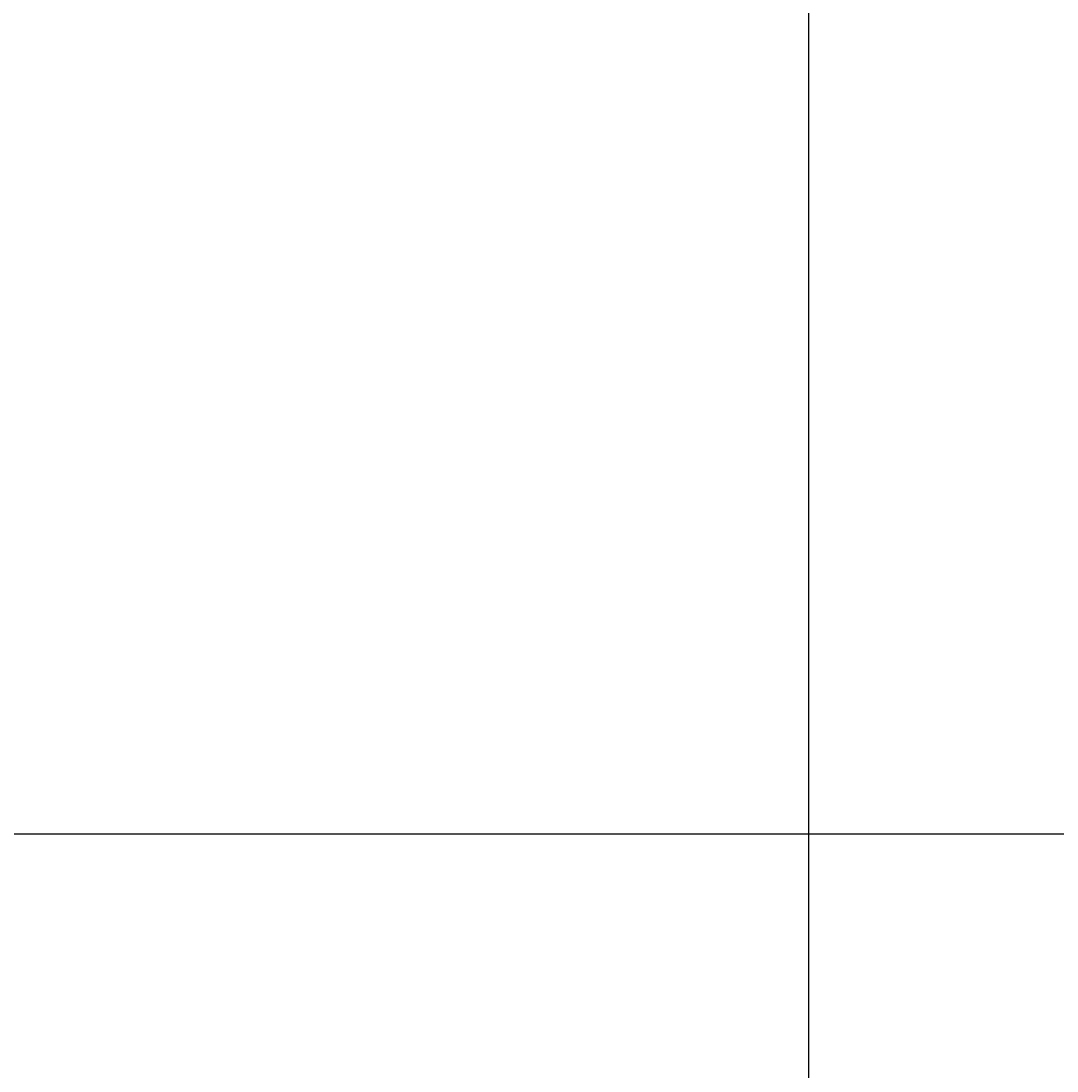
# Model space of a CAD drawing. Units: inches. Extents: x 35362 to 73946, y 43607 to 67532.
# Tile 50 of 134: x 49302 to 50119, y 45263 to 46091. Entities that reach past the tile are written whole.
import ezdxf

# ---------------------------------------------------------------- set-up
doc = ezdxf.new("R2010")
doc.units = ezdxf.units.IN
doc.header["$MEASUREMENT"] = 0
doc.layers.add('A-ANNO-DIMS', color=2, linetype='Continuous', lineweight=18)
doc.styles.get("Standard").update_dxf_attribs({"font": 'arial.ttf'})
doc.dimstyles.get("Standard").update_dxf_attribs({"dimtxt": 0.18, "dimasz": 0.18, "dimexe": 0.18, "dimexo": 0.0625, "dimgap": 0.09, "dimtad": 0, "dimtih": 1, "dimtoh": 1, "dimdec": 4, "dimzin": 0, "dimdsep": 46, "dimtxsty": 'Standard', "dimcen": 0.09, "dimadec": 0, "dimazin": 0, "dimtfac": 1, "dimtdec": 4, "dimtofl": 0, "dimtmove": 0, "dimatfit": 3, "dimfxl": 1, "dimtolj": 1, "dimtzin": 0, "dimarcsym": 0})

# ---------------------------------------------------------------- blocks, each defined once
blk = doc.blocks.new('*D5')
at = {"layer": 'A-ANNO-DIMS', "color": 0, "lineweight": -2, "transparency": 16777216}
for p, q in [((37121.95, 46919.32), (37121.95, 43606.68)), ((69871.5, 45449.83), (69871.5, 43606.68)), ((37122.13, 43606.86), (53496.29, 43606.86)), ((69871.32, 43606.86), (53497.15, 43606.86))]:
    blk.add_line(p, q, dxfattribs=at)
at = {"layer": 'A-ANNO-DIMS', "color": 0, "transparency": 16777216}
for points in [[(37122.13, 43606.89), (37122.13, 43606.83), (37121.95, 43606.86)], [(69871.32, 43606.89), (69871.32, 43606.83), (69871.5, 43606.86)]]:
    blk.add_solid(points, dxfattribs=at)
at = {"layer": 'Defpoints', "color": 0, "transparency": 16777216}
for p in [(37121.95, 46919.38), (69871.5, 45449.89), (69871.5, 43606.86)]:
    blk.add_point(p, dxfattribs=at)
at = {"layer": 'A-ANNO-DIMS', "color": 0, "transparency": 16777216, "insert": (53496.72, 43606.86), "char_height": 0.18, "attachment_point": 5}
blk.add_mtext('\\A1;32750', dxfattribs=at)
blk = doc.blocks.new('*D11')
at = {"layer": 'A-ANNO-DIMS', "color": 0, "lineweight": -2, "transparency": 16777216}
for p, q in [((47978.66, 56028.77), (47978.66, 43606.68)), ((53109.76, 56028.77), (53109.76, 43606.68)), ((47978.84, 43606.86), (50543.87, 43606.86)), ((53109.58, 43606.86), (50544.55, 43606.86))]:
    blk.add_line(p, q, dxfattribs=at)
at = {"layer": 'A-ANNO-DIMS', "color": 0, "transparency": 16777216}
for points in [[(47978.84, 43606.89), (47978.84, 43606.83), (47978.66, 43606.86)], [(53109.58, 43606.89), (53109.58, 43606.83), (53109.76, 43606.86)]]:
    blk.add_solid(points, dxfattribs=at)
at = {"layer": 'Defpoints', "color": 0, "transparency": 16777216}
for p in [(47978.66, 56028.84), (53109.76, 56028.84), (53109.76, 43606.86)]:
    blk.add_point(p, dxfattribs=at)
at = {"layer": 'A-ANNO-DIMS', "color": 0, "transparency": 16777216, "insert": (50544.21, 43606.86), "char_height": 0.18, "attachment_point": 5}
blk.add_mtext('\\A1;5131', dxfattribs=at)
blk = doc.blocks.new('*D13')
at = {"layer": 'A-ANNO-DIMS', "color": 0, "lineweight": -2, "transparency": 16777216}
for p, q in [((48373.49, 51694.02), (48373.49, 43606.68)), ((51029.04, 51694.02), (51029.04, 43606.68)), ((48373.67, 43606.86), (49700.8, 43606.86)), ((51028.86, 43606.86), (49701.73, 43606.86))]:
    blk.add_line(p, q, dxfattribs=at)
at = {"layer": 'A-ANNO-DIMS', "color": 0, "transparency": 16777216}
for points in [[(48373.67, 43606.89), (48373.67, 43606.83), (48373.49, 43606.86)], [(51028.86, 43606.89), (51028.86, 43606.83), (51029.04, 43606.86)]]:
    blk.add_solid(points, dxfattribs=at)
at = {"layer": 'Defpoints', "color": 0, "transparency": 16777216}
for p in [(48373.49, 51694.09), (51029.04, 51694.09), (51029.04, 43606.86)]:
    blk.add_point(p, dxfattribs=at)
at = {"layer": 'A-ANNO-DIMS', "color": 0, "transparency": 16777216, "insert": (49701.27, 43606.86), "char_height": 0.18, "attachment_point": 5}
blk.add_mtext('\\A1;2655.6', dxfattribs=at)
blk = doc.blocks.new('*D17')
at = {"layer": 'A-ANNO-DIMS', "color": 0, "lineweight": -2, "transparency": 16777216}
for p, q in [((49923.31, 61293.22), (49923.31, 43606.68)), ((51913.93, 61293.22), (51913.93, 43606.68)), ((49923.49, 43606.86), (50918.16, 43606.86)), ((51913.75, 43606.86), (50919.07, 43606.86))]:
    blk.add_line(p, q, dxfattribs=at)
at = {"layer": 'A-ANNO-DIMS', "color": 0, "transparency": 16777216}
for points in [[(49923.49, 43606.89), (49923.49, 43606.83), (49923.31, 43606.86)], [(51913.75, 43606.89), (51913.75, 43606.83), (51913.93, 43606.86)]]:
    blk.add_solid(points, dxfattribs=at)
at = {"layer": 'Defpoints', "color": 0, "transparency": 16777216}
for p in [(49923.31, 61293.29), (51913.93, 61293.29), (51913.93, 43606.86)]:
    blk.add_point(p, dxfattribs=at)
at = {"layer": 'A-ANNO-DIMS', "color": 0, "transparency": 16777216, "insert": (50918.62, 43606.86), "char_height": 0.18, "attachment_point": 5}
blk.add_mtext('\\A1;1990.6', dxfattribs=at)
blk = doc.blocks.new('*D67')
at = {"layer": 'A-ANNO-DIMS', "color": 0, "lineweight": -2, "transparency": 16777216}
for p, q in [((56873.54, 53351.53), (35361.77, 53351.53)), ((35361.95, 53351.35), (35361.95, 49400.89)), ((35361.95, 45450.07), (35361.95, 49400.53)), ((53793.58, 45449.89), (35361.77, 45449.89))]:
    blk.add_line(p, q, dxfattribs=at)
at = {"layer": 'A-ANNO-DIMS', "color": 0, "transparency": 16777216}
for points in [[(35361.92, 53351.35), (35361.98, 53351.35), (35361.95, 53351.53)], [(35361.92, 45450.07), (35361.98, 45450.07), (35361.95, 45449.89)]]:
    blk.add_solid(points, dxfattribs=at)
at = {"layer": 'Defpoints', "color": 0, "transparency": 16777216}
for p in [(35361.95, 53351.53), (56873.6, 53351.53), (53793.64, 45449.89)]:
    blk.add_point(p, dxfattribs=at)
at = {"layer": 'A-ANNO-DIMS', "color": 0, "transparency": 16777216, "insert": (35361.95, 49400.71), "char_height": 0.18, "attachment_point": 5}
blk.add_mtext('\\A1;7901.6', dxfattribs=at)

msp = doc.modelspace()

# ---------------------------------------------------------------- dimensions: what is measured, and where the dimension line sits
at = {"layer": 'A-ANNO-DIMS'}
for base, p1, p2, override, picture, middle in [((51913.931, 43606.859), (49923.307, 61293.286), (51913.931, 61293.286), {"dimdec": 1, "dimlfac": 1, "dimrnd": 0, "dimzin": 0, "dimdsep": 46, "dimlunit": 2}, '*D17', (50918.619, 43606.859)), ((53109.76, 43606.859), (47978.665, 56028.836), (53109.76, 56028.836), {"dimdec": 0, "dimlfac": 1, "dimrnd": 0, "dimzin": 0, "dimdsep": 46, "dimlunit": 2}, '*D11', (50544.212, 43606.859)), ((51029.043, 43606.859), (48373.492, 51694.087), (51029.043, 51694.087), {"dimdec": 1, "dimlfac": 1, "dimrnd": 0, "dimzin": 0, "dimdsep": 46, "dimlunit": 2}, '*D13', (49701.267, 43606.859)), ((69871.496, 43606.859), (37121.949, 46919.381), (69871.496, 45449.894), {"dimdec": 0, "dimlfac": 1, "dimrnd": 0, "dimzin": 0, "dimdsep": 46, "dimlunit": 2}, '*D5', (53496.723, 43606.859))]:
    dim = msp.add_linear_dim(base=base, p1=p1, p2=p2, dimstyle='Standard', override=override, dxfattribs=at)
    dim.commit()
    dim.dimension.update_dxf_attribs({"geometry": picture, "text_midpoint": middle})
dim = msp.add_linear_dim(base=(35361.949, 53351.529), p1=(53793.638, 45449.894), p2=(56873.602, 53351.529), angle=90, dimstyle='Standard', override={"dimdec": 1, "dimlfac": 1, "dimrnd": 0, "dimzin": 0, "dimdsep": 46, "dimlunit": 2}, dxfattribs=at)
dim.commit()
dim.dimension.update_dxf_attribs({"geometry": '*D67', "text_midpoint": (35361.949, 49400.712)})

doc.saveas('drawing.dxf')
